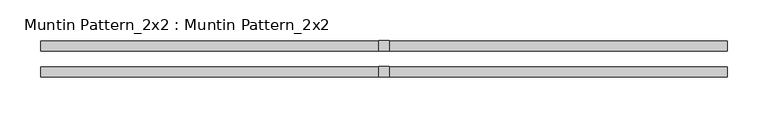
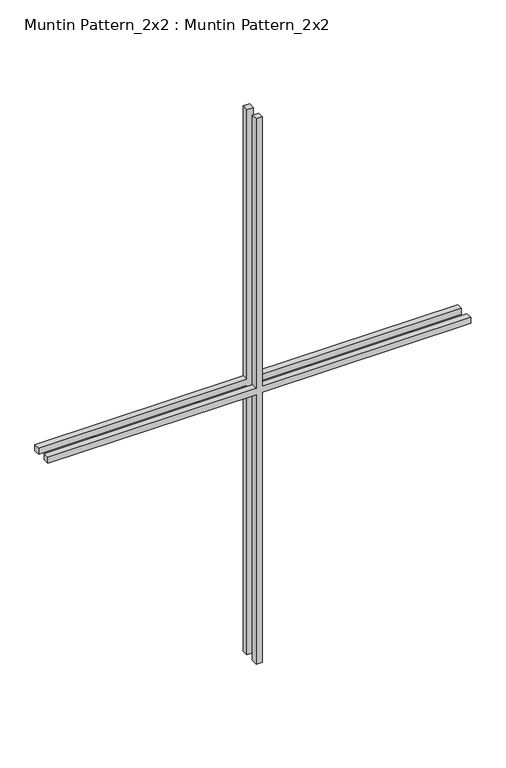
"""IFC4 building model written with IfcOpenShell, lengths in millimetres: proxy geometry, Muntin Pattern_2x2 : Muntin Pattern_2x2."""

from ifc_helpers import new_model, si_unit, frame, origin, place, context, project, spatial, polyline, outline, extrude, source, transform, mapped, element, save


def muntin_pattern_2x2_muntin_pattern_2x2_0b2f62cf(model_context):
    return source(origin(), model_context, "Body", "SweptSolid", [
        extrude(outline(polyline([(577.85, -6.35), (577.85, -419.1), (565.15, -419.1), (565.15, -6.35), (0.0, -6.35), (0.0, 6.35), (565.15, 6.35), (565.15, 419.1), (577.85, 419.1), (577.85, 6.35), (1143.0, 6.35), (1143.0, -6.35), (577.85, -6.35)])), frame((0.0, -22.225, 0.0), z_axis=(0.0, 1.0, 0.0), x_axis=(0.0, 0.0, 1.0)), (0.0, 0.0, 1.0), 12.7),
        extrude(outline(polyline([(577.85, -6.35), (577.85, -419.1), (565.15, -419.1), (565.15, -6.35), (0.0, -6.35), (0.0, 6.35), (565.15, 6.35), (565.15, 419.1), (577.85, 419.1), (577.85, 6.35), (1143.0, 6.35), (1143.0, -6.35), (577.85, -6.35)])), frame((0.0, 9.525, 0.0), z_axis=(0.0, 1.0, 0.0), x_axis=(0.0, 0.0, 1.0)), (0.0, 0.0, 1.0), 12.7),
    ])


if __name__ == "__main__":
    model = new_model("IFC4")
    model_context = context("Model", 3, world=origin())
    ifc_project = project(units=[si_unit("LENGTHUNIT", "METRE", prefix="MILLI")], contexts=[model_context])
    site = spatial("IfcSite", under=ifc_project)
    building = spatial("IfcBuilding", under=site)
    placement = place(None, origin())
    muntin_pattern_2x2_muntin_pattern_2x2_shape = muntin_pattern_2x2_muntin_pattern_2x2_0b2f62cf(model_context)
    element("IfcBuildingElementProxy", 1, Name="Muntin Pattern_2x2 : Muntin Pattern_2x2", ObjectType="Muntin Pattern_2x2 : Muntin Pattern_2x2", at=placement, inside=building, context=model_context, shape_type="MappedRepresentation", body=[
        mapped(muntin_pattern_2x2_muntin_pattern_2x2_shape, transform((0.0, 0.0, 0.0), x_axis=(1.0, 0.0, 0.0), y_axis=(0.0, 1.0, 0.0), z_axis=(0.0, 0.0, 1.0))),
    ])
    save(model, "model.ifc")

# Revit data of these elements
# Type "Muntin Pattern_2x2 : Muntin Pattern_2x2"
#   Width [instance default] = 4' - 0"
#   Thickness = 0' - 0 1/2"
#   Height [instance default] = 4' - 0"
#   Distance = 0' - 0 3/4"
#   Interior Material [instance default] = none
#   Exterior Material [instance default] = none
#   Default Elevation = 0
# Element 1 (IfcBuildingElementProxy, "Muntin Pattern_2x2 : Muntin Pattern_2x2")
#   Width = 2' - 9"
#   Height = 3' - 9"
#   Interior Material = Wood - Stained
#   Exterior Material = Clad - White
#   Materials on its faces: "Clad - White", "Wood - Stained"
# Materials
#   "Clad - White": class "Wood", colour RGB 242 242 238, transparency 0, Cost = 0
#   "Wood - Stained": class "Wood", colour RGB 224 178 126, transparency 0, Cost = 0
